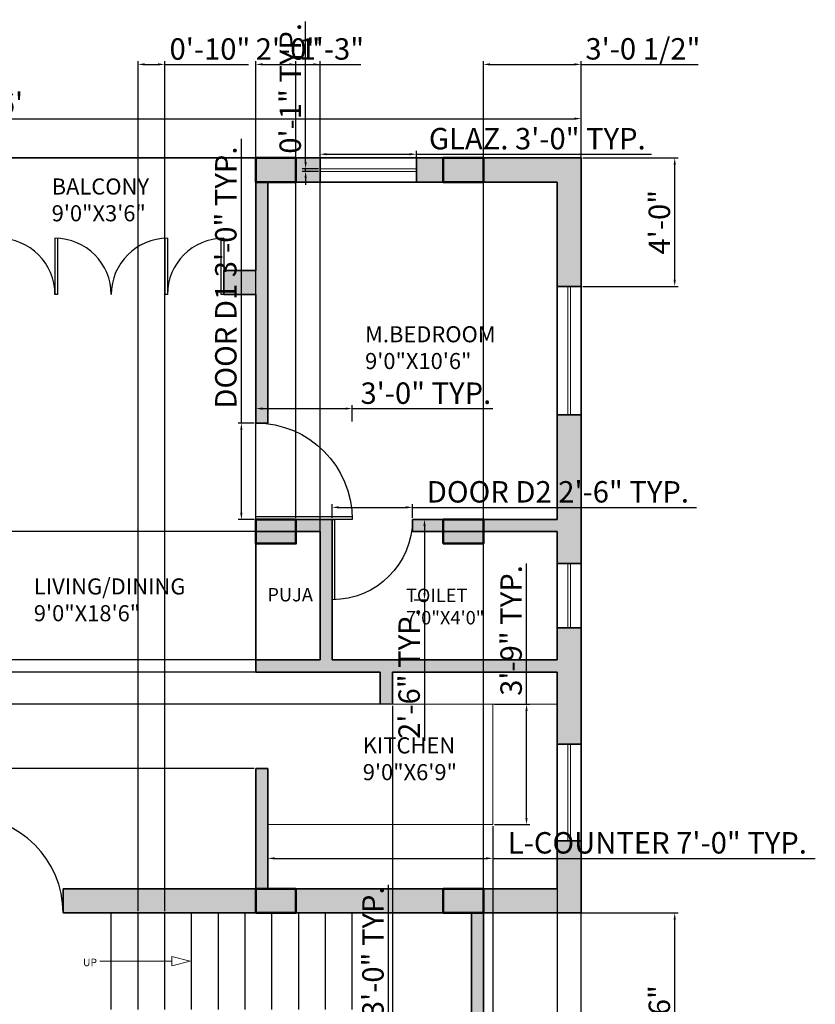
# Model space of a CAD drawing. Units: inches. Extents: x 3010 to 3575, y 2253 to 2995.
# Tile 4 of 4: x 3278 to 3575, y 2627 to 2995. Entities that reach past the tile are written whole.
import ezdxf

# ---------------------------------------------------------------- set-up
doc = ezdxf.new("R2010")
doc.units = ezdxf.units.IN
for name, color, linetype, lineweight in [('A-ANNO-DIMS', 2, 'Continuous', 18), ('A-ANNO-SYMB', 7, 'Continuous', 18), ('A-ANNO-TEXT', 7, 'Continuous', 18), ('A-AREA-IDEN', 7, 'Continuous', 18), ('A-COLS', 7, 'Continuous', 50), ('A-COLS-PATT', 1, 'Continuous', 13), ('A-DOOR', 3, 'Continuous', 25), ('A-FLOR-FIXT', 8, 'Continuous', 18), ('A-FLOR-STRS', 7, 'Continuous', 25), ('A-GLAZ', 4, 'Continuous', 18), ('A-WALL', 7, 'Continuous', 35)]:
    doc.layers.add(name, color=color, linetype=linetype, lineweight=lineweight)
doc.layers.add('A-WALL-PATT', color=9, linetype='Continuous', lineweight=13, true_color=0xc7c8ca)
doc.styles.get("Standard").update_dxf_attribs({"font": 'arial.ttf'})
doc.dimstyles.new('ISO-25', dxfattribs={"dimtxt": 8, "dimasz": 2.5, "dimexe": 1.25, "dimexo": 0.625, "dimtad": 1, "dimdec": 1, "dimlunit": 3, "dimtxsty": 'Standard', "dimcen": 2.5, "dimadec": 0, "dimazin": 0, "dimtfac": 1, "dimtdec": 1, "dimtmove": 0, "dimatfit": 3, "dimfxl": 1, "dimarcsym": 0})

# ---------------------------------------------------------------- blocks, each defined once
blk = doc.blocks.new('*D1')
at = {"layer": 'A-ANNO-DIMS', "color": 0, "lineweight": -2, "transparency": 16777216}
for p, q in [((3055.45, 2944.01), (3055.45, 2959.31)), ((3057.95, 2958.06), (3484.95, 2958.06)), ((3487.45, 2944.01), (3487.45, 2959.31))]:
    blk.add_line(p, q, dxfattribs=at)
at = {"layer": 'A-ANNO-DIMS', "color": 0, "transparency": 16777216}
for points in [[(3057.95, 2958.48), (3057.95, 2957.65), (3055.45, 2958.06)], [(3484.95, 2958.48), (3484.95, 2957.65), (3487.45, 2958.06)]]:
    blk.add_solid(points, dxfattribs=at)
at = {"layer": 'Defpoints', "color": 0, "transparency": 16777216}
for p in [(3487.45, 2958.06), (3055.45, 2943.38), (3487.45, 2943.38)]:
    blk.add_point(p, dxfattribs=at)
at = {"layer": 'A-ANNO-DIMS', "color": 0, "transparency": 16777216, "insert": (3271.45, 2962.78), "char_height": 8, "attachment_point": 5}
blk.add_mtext("36'", dxfattribs=at)
blk = doc.blocks.new("D2 2'6")
for p, q in [((0, 30), (0, 0)), ((1, 30), (1, 0)), ((0, 0), (1, 0))]:
    blk.add_line(p, q)
blk.add_arc((0, 0), 30, 0, 90)
blk = doc.blocks.new("D1 3'")
for p, q in [((0, 36), (0, 0)), ((1, 36), (1, 0)), ((0, 0), (1, 0))]:
    blk.add_line(p, q)
blk.add_arc((0, 0), 36, 0, 90)
blk = doc.blocks.new('FLOD D')
for p, q in [((3539.49, 2401.61), (3539.49, 2380.61)), ((3540.49, 2401.61), (3540.49, 2380.61)), ((3560.49, 2401.61), (3560.49, 2380.61)), ((3561.49, 2401.61), (3561.49, 2380.61)), ((3601.49, 2401.61), (3601.49, 2380.61)), ((3602.49, 2401.61), (3602.49, 2380.61)), ((3622.49, 2401.61), (3622.49, 2380.61)), ((3623.49, 2401.61), (3623.49, 2380.61)), ((3540.49, 2380.61), (3539.49, 2380.61)), ((3561.49, 2380.61), (3560.49, 2380.61)), ((3602.49, 2380.61), (3601.49, 2380.61)), ((3623.49, 2380.61), (3622.49, 2380.61))]:
    blk.add_line(p, q)
for centre, start, end in [((3539.49, 2380.61), 0, 90), ((3560.49, 2380.61), 0, 90), ((3602.49, 2380.61), 90, 180), ((3623.49, 2380.61), 90, 180)]:
    blk.add_arc(centre, 21, start, end)
blk = doc.blocks.new('GLAZING-24IN')
for p, q in [((24, 1), (0, 1)), ((24, 0), (0, 0))]:
    blk.add_line(p, q)
blk = doc.blocks.new('GLAZING-36IN')
for p, q in [((36, 1), (0, 1)), ((36, 0), (0, 0))]:
    blk.add_line(p, q)
blk = doc.blocks.new('GLAZING-48IN')
for p, q in [((48, 1), (0, 1)), ((48, 0), (0, 0))]:
    blk.add_line(p, q)
blk = doc.blocks.new('STAIR-FLIGHT-36IN')
for p, q in [((0, 0), (0, 36)), ((10, 0), (10, 36)), ((20, 0), (20, 36)), ((30, 0), (30, 36)), ((40, 0), (40, 36)), ((50, 0), (50, 36)), ((60, 0), (60, 36)), ((70, 0), (70, 36)), ((80, 0), (80, 36)), ((90, 0), (90, 36))]:
    blk.add_line(p, q)
blk = doc.blocks.new('STAIR-DIRECTION-ARROW')
blk.add_line((0, 1.77), (26.94, 1.77))
blk.add_lwpolyline([(33.73, 1.77), (26.94, 3.54), (26.94, 0)], close=True)
blk = doc.blocks.new('KITCHEN-COUNTER-L')
for p, q in [((84, 45), (84, 0)), ((84, 0), (0, 0))]:
    blk.add_line(p, q)
blk = doc.blocks.new('*D15')
at = {"layer": 'A-ANNO-DIMS', "color": 0, "lineweight": -2, "transparency": 16777216}
for p, q in [((3389.94, 2940.01), (3389.94, 2946.03)), ((3425.94, 2940.01), (3425.94, 2946.03)), ((3392.44, 2944.78), (3423.44, 2944.78)), ((3425.94, 2944.78), (3513.72, 2944.78))]:
    blk.add_line(p, q, dxfattribs=at)
at = {"layer": 'A-ANNO-DIMS', "color": 0, "transparency": 16777216}
for points in [[(3392.44, 2945.2), (3392.44, 2944.37), (3389.94, 2944.78)], [(3423.44, 2945.2), (3423.44, 2944.37), (3425.94, 2944.78)]]:
    blk.add_solid(points, dxfattribs=at)
at = {"layer": 'Defpoints', "color": 0, "transparency": 16777216}
for p in [(3425.94, 2944.78), (3389.94, 2939.38), (3425.94, 2939.38)]:
    blk.add_point(p, dxfattribs=at)
at = {"layer": 'A-ANNO-DIMS', "color": 0, "transparency": 16777216, "insert": (3471.08, 2949.55), "char_height": 8, "attachment_point": 5}
blk.add_mtext('GLAZ. 3\'-0" TYP.', dxfattribs=at)
blk = doc.blocks.new('*D16')
at = {"layer": 'A-ANNO-DIMS', "color": 0, "lineweight": -2, "transparency": 16777216}
for p, q in [((3384.54, 2941.88), (3384.54, 2994.4)), ((3389.31, 2939.38), (3383.29, 2939.38)), ((3389.31, 2938.38), (3383.29, 2938.38)), ((3384.54, 2938.38), (3384.54, 2939.38)), ((3384.54, 2935.88), (3384.54, 2933.38))]:
    blk.add_line(p, q, dxfattribs=at)
at = {"layer": 'A-ANNO-DIMS', "color": 0, "transparency": 16777216}
for points in [[(3384.12, 2941.88), (3384.95, 2941.88), (3384.54, 2939.38)], [(3384.12, 2935.88), (3384.95, 2935.88), (3384.54, 2938.38)]]:
    blk.add_solid(points, dxfattribs=at)
at = {"layer": 'Defpoints', "color": 0, "transparency": 16777216}
for p in [(3384.54, 2939.38), (3389.94, 2939.38), (3389.94, 2938.38)]:
    blk.add_point(p, dxfattribs=at)
at = {"layer": 'A-ANNO-DIMS', "color": 0, "transparency": 16777216, "insert": (3379.83, 2969.39), "char_height": 8, "attachment_point": 5, "rotation": 90}
blk.add_mtext('0\'-1" TYP.', dxfattribs=at)
blk = doc.blocks.new('*D23')
at = {"layer": 'A-ANNO-DIMS', "color": 0, "lineweight": -2, "transparency": 16777216}
for p, q in [((3360.55, 2844.38), (3360.55, 2950.52)), ((3365.32, 2844.38), (3359.3, 2844.38)), ((3360.55, 2810.88), (3360.55, 2841.88)), ((3365.32, 2808.38), (3359.3, 2808.38))]:
    blk.add_line(p, q, dxfattribs=at)
at = {"layer": 'A-ANNO-DIMS', "color": 0, "transparency": 16777216}
for points in [[(3360.13, 2841.88), (3360.96, 2841.88), (3360.55, 2844.38)], [(3360.13, 2810.88), (3360.96, 2810.88), (3360.55, 2808.38)]]:
    blk.add_solid(points, dxfattribs=at)
at = {"layer": 'Defpoints', "color": 0, "transparency": 16777216}
for p in [(3360.55, 2844.38), (3365.95, 2844.38), (3365.95, 2808.38)]:
    blk.add_point(p, dxfattribs=at)
at = {"layer": 'A-ANNO-DIMS', "color": 0, "transparency": 16777216, "insert": (3355.78, 2898.7), "char_height": 8, "attachment_point": 5, "rotation": 90}
blk.add_mtext('DOOR D1 3\'-0" TYP.', dxfattribs=at)
blk = doc.blocks.new('*D24')
at = {"layer": 'A-ANNO-DIMS', "color": 0, "lineweight": -2, "transparency": 16777216}
for p, q in [((3365.95, 2845.01), (3365.95, 2851.03)), ((3401.95, 2845.01), (3401.95, 2851.03)), ((3368.45, 2849.78), (3399.45, 2849.78)), ((3401.95, 2849.78), (3454.45, 2849.78))]:
    blk.add_line(p, q, dxfattribs=at)
at = {"layer": 'A-ANNO-DIMS', "color": 0, "transparency": 16777216}
for points in [[(3368.45, 2850.2), (3368.45, 2849.37), (3365.95, 2849.78)], [(3399.45, 2850.2), (3399.45, 2849.37), (3401.95, 2849.78)]]:
    blk.add_solid(points, dxfattribs=at)
at = {"layer": 'Defpoints', "color": 0, "transparency": 16777216}
for p in [(3401.95, 2849.78), (3365.95, 2844.38), (3401.95, 2844.38)]:
    blk.add_point(p, dxfattribs=at)
at = {"layer": 'A-ANNO-DIMS', "color": 0, "transparency": 16777216, "insert": (3429.45, 2854.5), "char_height": 8, "attachment_point": 5}
blk.add_mtext('3\'-0" TYP.', dxfattribs=at)
blk = doc.blocks.new('*D25')
at = {"layer": 'A-ANNO-DIMS', "color": 0, "lineweight": -2, "transparency": 16777216}
for p, q in [((3394.45, 2809.01), (3394.45, 2814.13)), ((3424.45, 2809.01), (3424.45, 2814.13)), ((3396.95, 2812.88), (3421.95, 2812.88)), ((3424.45, 2812.88), (3530.59, 2812.88))]:
    blk.add_line(p, q, dxfattribs=at)
at = {"layer": 'A-ANNO-DIMS', "color": 0, "transparency": 16777216}
for points in [[(3396.95, 2813.3), (3396.95, 2812.47), (3394.45, 2812.88)], [(3421.95, 2813.3), (3421.95, 2812.47), (3424.45, 2812.88)]]:
    blk.add_solid(points, dxfattribs=at)
at = {"layer": 'Defpoints', "color": 0, "transparency": 16777216}
for p in [(3424.45, 2812.88), (3394.45, 2808.38), (3424.45, 2808.38)]:
    blk.add_point(p, dxfattribs=at)
at = {"layer": 'A-ANNO-DIMS', "color": 0, "transparency": 16777216, "insert": (3478.77, 2817.65), "char_height": 8, "attachment_point": 5}
blk.add_mtext('DOOR D2 2\'-6" TYP.', dxfattribs=at)
blk = doc.blocks.new('*D26')
at = {"layer": 'A-ANNO-DIMS', "color": 0, "lineweight": -2, "transparency": 16777216}
for p, q in [((3425.07, 2808.38), (3430.2, 2808.38)), ((3428.95, 2805.88), (3428.95, 2780.88)), ((3425.07, 2778.38), (3430.2, 2778.38)), ((3428.95, 2778.38), (3428.95, 2725.73))]:
    blk.add_line(p, q, dxfattribs=at)
at = {"layer": 'A-ANNO-DIMS', "color": 0, "transparency": 16777216}
for points in [[(3428.53, 2805.88), (3429.36, 2805.88), (3428.95, 2808.38)], [(3428.53, 2780.88), (3429.36, 2780.88), (3428.95, 2778.38)]]:
    blk.add_solid(points, dxfattribs=at)
at = {"layer": 'Defpoints', "color": 0, "transparency": 16777216}
for p in [(3424.45, 2808.38), (3424.45, 2778.38), (3428.95, 2778.38)]:
    blk.add_point(p, dxfattribs=at)
at = {"layer": 'A-ANNO-DIMS', "color": 0, "transparency": 16777216, "insert": (3424.24, 2750.81), "char_height": 8, "attachment_point": 5, "rotation": 90}
blk.add_mtext('2\'-6" TYP.', dxfattribs=at)
blk = doc.blocks.new('*D31')
at = {"layer": 'A-ANNO-DIMS', "color": 0, "lineweight": -2, "transparency": 16777216}
for p, q in [((3370.45, 2693.76), (3370.45, 2680.53)), ((3454.45, 2693.76), (3454.45, 2680.53)), ((3372.95, 2681.78), (3451.95, 2681.78)), ((3454.45, 2681.78), (3574.9, 2681.78))]:
    blk.add_line(p, q, dxfattribs=at)
at = {"layer": 'A-ANNO-DIMS', "color": 0, "transparency": 16777216}
for points in [[(3372.95, 2682.2), (3372.95, 2681.37), (3370.45, 2681.78)], [(3451.95, 2682.2), (3451.95, 2681.37), (3454.45, 2681.78)]]:
    blk.add_solid(points, dxfattribs=at)
at = {"layer": 'Defpoints', "color": 0, "transparency": 16777216}
for p in [(3370.45, 2694.38), (3454.45, 2694.38), (3454.45, 2681.78)]:
    blk.add_point(p, dxfattribs=at)
at = {"layer": 'A-ANNO-DIMS', "color": 0, "transparency": 16777216, "insert": (3515.92, 2686.55), "char_height": 8, "attachment_point": 5}
blk.add_mtext('L-COUNTER 7\'-0" TYP.', dxfattribs=at)
blk = doc.blocks.new('*D32')
at = {"layer": 'A-ANNO-DIMS', "color": 0, "lineweight": -2, "transparency": 16777216}
for p, q in [((3467.05, 2739.38), (3467.05, 2791.89)), ((3455.07, 2739.38), (3468.3, 2739.38)), ((3467.05, 2696.88), (3467.05, 2736.88)), ((3455.07, 2694.38), (3468.3, 2694.38))]:
    blk.add_line(p, q, dxfattribs=at)
at = {"layer": 'A-ANNO-DIMS', "color": 0, "transparency": 16777216}
for points in [[(3466.63, 2736.88), (3467.46, 2736.88), (3467.05, 2739.38)], [(3466.63, 2696.88), (3467.46, 2696.88), (3467.05, 2694.38)]]:
    blk.add_solid(points, dxfattribs=at)
at = {"layer": 'Defpoints', "color": 0, "transparency": 16777216}
for p in [(3454.45, 2739.38), (3467.05, 2739.38), (3454.45, 2694.38)]:
    blk.add_point(p, dxfattribs=at)
at = {"layer": 'A-ANNO-DIMS', "color": 0, "transparency": 16777216, "insert": (3462.33, 2766.89), "char_height": 8, "attachment_point": 5, "rotation": 90}
blk.add_mtext('3\'-9" TYP.', dxfattribs=at)
blk = doc.blocks.new('*D34')
at = {"layer": 'A-ANNO-DIMS', "color": 0, "lineweight": -2, "transparency": 16777216}
for p, q in [((3415.45, 2619.38), (3415.45, 2671.89)), ((3402.57, 2619.38), (3416.7, 2619.38)), ((3415.45, 2585.88), (3415.45, 2616.88)), ((3402.57, 2583.38), (3416.7, 2583.38))]:
    blk.add_line(p, q, dxfattribs=at)
at = {"layer": 'A-ANNO-DIMS', "color": 0, "transparency": 16777216}
for points in [[(3415.03, 2616.88), (3415.86, 2616.88), (3415.45, 2619.38)], [(3415.03, 2585.88), (3415.86, 2585.88), (3415.45, 2583.38)]]:
    blk.add_solid(points, dxfattribs=at)
at = {"layer": 'Defpoints', "color": 0, "transparency": 16777216}
for p in [(3401.95, 2619.38), (3415.45, 2619.38), (3401.95, 2583.38)]:
    blk.add_point(p, dxfattribs=at)
at = {"layer": 'A-ANNO-DIMS', "color": 0, "transparency": 16777216, "insert": (3410.73, 2646.89), "char_height": 8, "attachment_point": 5, "rotation": 90}
blk.add_mtext('3\'-0" TYP.', dxfattribs=at)
blk = doc.blocks.new('*D37')
at = {"layer": 'A-ANNO-DIMS', "color": 0, "lineweight": -2, "transparency": 16777216}
for p, q in [((3447.07, 2661.38), (3523.65, 2661.38)), ((3522.4, 2585.88), (3522.4, 2658.88)), ((3447.07, 2583.38), (3523.65, 2583.38))]:
    blk.add_line(p, q, dxfattribs=at)
at = {"layer": 'A-ANNO-DIMS', "color": 0, "transparency": 16777216}
for points in [[(3521.98, 2658.88), (3522.81, 2658.88), (3522.4, 2661.38)], [(3521.98, 2585.88), (3522.81, 2585.88), (3522.4, 2583.38)]]:
    blk.add_solid(points, dxfattribs=at)
at = {"layer": 'Defpoints', "color": 0, "transparency": 16777216}
for p in [(3446.45, 2661.38), (3522.4, 2661.38), (3446.45, 2583.38)]:
    blk.add_point(p, dxfattribs=at)
at = {"layer": 'A-ANNO-DIMS', "color": 0, "transparency": 16777216, "insert": (3517.69, 2622.38), "char_height": 8, "attachment_point": 5, "rotation": 90}
blk.add_mtext('6\'-6"', dxfattribs=at)
blk = doc.blocks.new('*D38')
at = {"layer": 'A-ANNO-DIMS', "color": 0, "lineweight": -2, "transparency": 16777216}
for p, q in [((3321.95, 2662.01), (3321.95, 2979.58)), ((3331.95, 2662.01), (3331.95, 2979.58)), ((3324.45, 2978.33), (3329.45, 2978.33)), ((3331.95, 2978.33), (3363.18, 2978.33))]:
    blk.add_line(p, q, dxfattribs=at)
at = {"layer": 'A-ANNO-DIMS', "color": 0, "transparency": 16777216}
for points in [[(3324.45, 2978.75), (3324.45, 2977.92), (3321.95, 2978.33)], [(3329.45, 2978.75), (3329.45, 2977.92), (3331.95, 2978.33)]]:
    blk.add_solid(points, dxfattribs=at)
at = {"layer": 'Defpoints', "color": 0, "transparency": 16777216}
for p in [(3331.95, 2978.33), (3321.95, 2661.38), (3331.95, 2661.38)]:
    blk.add_point(p, dxfattribs=at)
at = {"layer": 'A-ANNO-DIMS', "color": 0, "transparency": 16777216, "insert": (3348.81, 2983.04), "char_height": 8, "attachment_point": 5}
blk.add_mtext('0\'-10"', dxfattribs=at)
blk = doc.blocks.new('*D39')
at = {"layer": 'A-ANNO-DIMS', "color": 0, "lineweight": -2, "transparency": 16777216}
for p, q in [((3365.95, 2756.51), (3365.95, 2979.58)), ((3389.95, 2756.51), (3389.95, 2979.58)), ((3368.45, 2978.33), (3387.45, 2978.33))]:
    blk.add_line(p, q, dxfattribs=at)
at = {"layer": 'A-ANNO-DIMS', "color": 0, "transparency": 16777216}
for points in [[(3368.45, 2978.75), (3368.45, 2977.92), (3365.95, 2978.33)], [(3387.45, 2978.75), (3387.45, 2977.92), (3389.95, 2978.33)]]:
    blk.add_solid(points, dxfattribs=at)
at = {"layer": 'Defpoints', "color": 0, "transparency": 16777216}
for p in [(3389.95, 2978.33), (3365.95, 2755.88), (3389.95, 2755.88)]:
    blk.add_point(p, dxfattribs=at)
at = {"layer": 'A-ANNO-DIMS', "color": 0, "transparency": 16777216, "insert": (3377.95, 2983.04), "char_height": 8, "attachment_point": 5}
blk.add_mtext('2\'-0"', dxfattribs=at)
blk = doc.blocks.new('*D40')
at = {"layer": 'A-ANNO-DIMS', "color": 0, "lineweight": -2, "transparency": 16777216}
for p, q in [((3389.32, 2803.88), (3019.25, 2803.88)), ((3020.5, 2758.38), (3020.5, 2801.38)), ((3389.32, 2755.88), (3019.25, 2755.88))]:
    blk.add_line(p, q, dxfattribs=at)
at = {"layer": 'A-ANNO-DIMS', "color": 0, "transparency": 16777216}
for points in [[(3020.08, 2801.38), (3020.91, 2801.38), (3020.5, 2803.88)], [(3020.08, 2758.38), (3020.91, 2758.38), (3020.5, 2755.88)]]:
    blk.add_solid(points, dxfattribs=at)
at = {"layer": 'Defpoints', "color": 0, "transparency": 16777216}
for p in [(3020.5, 2803.88), (3389.95, 2803.88), (3389.95, 2755.88)]:
    blk.add_point(p, dxfattribs=at)
at = {"layer": 'A-ANNO-DIMS', "color": 0, "transparency": 16777216, "insert": (3015.79, 2779.88), "char_height": 8, "attachment_point": 5, "rotation": 90}
blk.add_mtext('4\'-0"', dxfattribs=at)
blk = doc.blocks.new('*D41')
at = {"layer": 'A-ANNO-DIMS', "color": 0, "lineweight": -2, "transparency": 16777216}
for p, q in [((3454.45, 2693.76), (3454.45, 2259.18)), ((3478.45, 2669.76), (3478.45, 2259.18)), ((3456.95, 2260.43), (3475.95, 2260.43))]:
    blk.add_line(p, q, dxfattribs=at)
at = {"layer": 'A-ANNO-DIMS', "color": 0, "transparency": 16777216}
for points in [[(3456.95, 2260.85), (3456.95, 2260.02), (3454.45, 2260.43)], [(3475.95, 2260.85), (3475.95, 2260.02), (3478.45, 2260.43)]]:
    blk.add_solid(points, dxfattribs=at)
at = {"layer": 'Defpoints', "color": 0, "transparency": 16777216}
for p in [(3454.45, 2694.38), (3478.45, 2670.38), (3478.45, 2260.43)]:
    blk.add_point(p, dxfattribs=at)
at = {"layer": 'A-ANNO-DIMS', "color": 0, "transparency": 16777216, "insert": (3466.45, 2265.14), "char_height": 8, "attachment_point": 5}
blk.add_mtext('2\'-0"', dxfattribs=at)
blk = doc.blocks.new('*D42')
at = {"layer": 'A-ANNO-DIMS', "color": 0, "lineweight": -2, "transparency": 16777216}
for p, q in [((3365.32, 2751.38), (3019.25, 2751.38)), ((3020.5, 2717.88), (3020.5, 2748.88)), ((3365.32, 2715.38), (3019.25, 2715.38))]:
    blk.add_line(p, q, dxfattribs=at)
at = {"layer": 'A-ANNO-DIMS', "color": 0, "transparency": 16777216}
for points in [[(3020.08, 2748.88), (3020.91, 2748.88), (3020.5, 2751.38)], [(3020.08, 2717.88), (3020.91, 2717.88), (3020.5, 2715.38)]]:
    blk.add_solid(points, dxfattribs=at)
at = {"layer": 'Defpoints', "color": 0, "transparency": 16777216}
for p in [(3020.5, 2751.38), (3365.95, 2751.38), (3365.95, 2715.38)]:
    blk.add_point(p, dxfattribs=at)
at = {"layer": 'A-ANNO-DIMS', "color": 0, "transparency": 16777216, "insert": (3015.78, 2733.38), "char_height": 8, "attachment_point": 5, "rotation": 90}
blk.add_mtext('3\'-0"', dxfattribs=at)
blk = doc.blocks.new('*D43')
at = {"layer": 'A-ANNO-DIMS', "color": 0, "lineweight": -2, "transparency": 16777216}
for p, q in [((3020.5, 2751.38), (3020.5, 2775.65)), ((3411.82, 2751.38), (3019.25, 2751.38)), ((3020.5, 2741.88), (3020.5, 2748.88)), ((3416.32, 2739.38), (3019.25, 2739.38))]:
    blk.add_line(p, q, dxfattribs=at)
at = {"layer": 'A-ANNO-DIMS', "color": 0, "transparency": 16777216}
for points in [[(3020.08, 2748.88), (3020.91, 2748.88), (3020.5, 2751.38)], [(3020.08, 2741.88), (3020.91, 2741.88), (3020.5, 2739.38)]]:
    blk.add_solid(points, dxfattribs=at)
at = {"layer": 'Defpoints', "color": 0, "transparency": 16777216}
for p in [(3020.5, 2751.38), (3412.45, 2751.38), (3416.95, 2739.38)]:
    blk.add_point(p, dxfattribs=at)
at = {"layer": 'A-ANNO-DIMS', "color": 0, "transparency": 16777216, "insert": (3015.79, 2764.76), "char_height": 8, "attachment_point": 5, "rotation": 90}
blk.add_mtext('1\'-0"', dxfattribs=at)
blk = doc.blocks.new('*D44')
at = {"layer": 'A-ANNO-DIMS', "color": 0, "lineweight": -2, "transparency": 16777216}
for p, q in [((3416.95, 2738.76), (3416.95, 2259.18)), ((3478.45, 2738.76), (3478.45, 2259.18)), ((3419.45, 2260.43), (3475.95, 2260.43))]:
    blk.add_line(p, q, dxfattribs=at)
at = {"layer": 'A-ANNO-DIMS', "color": 0, "transparency": 16777216}
for points in [[(3419.45, 2260.85), (3419.45, 2260.02), (3416.95, 2260.43)], [(3475.95, 2260.85), (3475.95, 2260.02), (3478.45, 2260.43)]]:
    blk.add_solid(points, dxfattribs=at)
at = {"layer": 'Defpoints', "color": 0, "transparency": 16777216}
for p in [(3416.95, 2739.38), (3478.45, 2739.38), (3478.45, 2260.43)]:
    blk.add_point(p, dxfattribs=at)
at = {"layer": 'A-ANNO-DIMS', "color": 0, "transparency": 16777216, "insert": (3447.7, 2265.19), "char_height": 8, "attachment_point": 5}
blk.add_mtext('5\'-1 1/2"', dxfattribs=at)
blk = doc.blocks.new('*D45')
at = {"layer": 'A-ANNO-DIMS', "color": 0, "lineweight": -2, "transparency": 16777216}
for p, q in [((3365.95, 2809.01), (3365.95, 2979.58)), ((3380.95, 2809.01), (3380.95, 2979.58)), ((3368.45, 2978.33), (3378.45, 2978.33)), ((3380.95, 2978.33), (3405.21, 2978.33))]:
    blk.add_line(p, q, dxfattribs=at)
at = {"layer": 'A-ANNO-DIMS', "color": 0, "transparency": 16777216}
for points in [[(3368.45, 2978.75), (3368.45, 2977.92), (3365.95, 2978.33)], [(3378.45, 2978.75), (3378.45, 2977.92), (3380.95, 2978.33)]]:
    blk.add_solid(points, dxfattribs=at)
at = {"layer": 'Defpoints', "color": 0, "transparency": 16777216}
for p in [(3380.95, 2978.33), (3365.95, 2808.38), (3380.95, 2808.38)]:
    blk.add_point(p, dxfattribs=at)
at = {"layer": 'A-ANNO-DIMS', "color": 0, "transparency": 16777216, "insert": (3394.33, 2983.05), "char_height": 8, "attachment_point": 5}
blk.add_mtext('1\'-3"', dxfattribs=at)
blk = doc.blocks.new('*D50')
at = {"layer": 'A-ANNO-DIMS', "color": 0, "lineweight": -2, "transparency": 16777216}
for p, q in [((3450.95, 2584.01), (3450.95, 2979.58)), ((3487.45, 2584.01), (3487.45, 2979.58)), ((3453.45, 2978.33), (3484.95, 2978.33)), ((3487.45, 2978.33), (3531.1, 2978.33))]:
    blk.add_line(p, q, dxfattribs=at)
at = {"layer": 'A-ANNO-DIMS', "color": 0, "transparency": 16777216}
for points in [[(3453.45, 2978.75), (3453.45, 2977.92), (3450.95, 2978.33)], [(3484.95, 2978.75), (3484.95, 2977.92), (3487.45, 2978.33)]]:
    blk.add_solid(points, dxfattribs=at)
at = {"layer": 'Defpoints', "color": 0, "transparency": 16777216}
for p in [(3487.45, 2978.33), (3450.95, 2583.38), (3487.45, 2583.38)]:
    blk.add_point(p, dxfattribs=at)
at = {"layer": 'A-ANNO-DIMS', "color": 0, "transparency": 16777216, "insert": (3510.52, 2983.1), "char_height": 8, "attachment_point": 5}
blk.add_mtext('3\'-0 1/2"', dxfattribs=at)
blk = doc.blocks.new('*D54')
at = {"layer": 'A-ANNO-DIMS', "color": 0, "lineweight": -2, "transparency": 16777216}
for p, q in [((3488.07, 2943.38), (3523.65, 2943.38)), ((3522.4, 2897.88), (3522.4, 2940.88)), ((3488.07, 2895.38), (3523.65, 2895.38))]:
    blk.add_line(p, q, dxfattribs=at)
at = {"layer": 'A-ANNO-DIMS', "color": 0, "transparency": 16777216}
for points in [[(3521.98, 2940.88), (3522.81, 2940.88), (3522.4, 2943.38)], [(3521.98, 2897.88), (3522.81, 2897.88), (3522.4, 2895.38)]]:
    blk.add_solid(points, dxfattribs=at)
at = {"layer": 'Defpoints', "color": 0, "transparency": 16777216}
for p in [(3487.45, 2943.38), (3522.4, 2943.38), (3487.45, 2895.38)]:
    blk.add_point(p, dxfattribs=at)
at = {"layer": 'A-ANNO-DIMS', "color": 0, "transparency": 16777216, "insert": (3517.69, 2919.38), "char_height": 8, "attachment_point": 5, "rotation": 90}
blk.add_mtext('4\'-0"', dxfattribs=at)

msp = doc.modelspace()

# ---------------------------------------------------------------- hatches: boundary and pattern name
at = {"layer": 'A-COLS-PATT'}
h = msp.add_hatch(color=256, dxfattribs=at)
h.dxf.hatch_style = 1
h.paths.add_polyline_path([(3380.95, 2934.38), (3380.95, 2943.38), (3365.95, 2943.38), (3365.95, 2934.38)])
h = msp.add_hatch(color=256, dxfattribs=at)
h.dxf.hatch_style = 1
h.paths.add_polyline_path([(3450.95, 2934.38), (3450.95, 2943.38), (3435.95, 2943.38), (3435.95, 2934.38)])
h = msp.add_hatch(color=256, dxfattribs=at)
h.dxf.hatch_style = 1
h.paths.add_polyline_path([(3380.95, 2799.38), (3380.95, 2808.38), (3365.95, 2808.38), (3365.95, 2799.38)])
h = msp.add_hatch(color=256, dxfattribs=at)
h.dxf.hatch_style = 1
h.paths.add_polyline_path([(3450.95, 2799.38), (3450.95, 2808.38), (3435.95, 2808.38), (3435.95, 2799.38)])
h = msp.add_hatch(color=256, dxfattribs=at)
h.dxf.hatch_style = 1
h.paths.add_polyline_path([(3380.95, 2661.38), (3380.95, 2670.38), (3365.95, 2670.38), (3365.95, 2661.38)])
h = msp.add_hatch(color=256, dxfattribs=at)
h.dxf.hatch_style = 1
h.paths.add_polyline_path([(3450.95, 2661.38), (3450.95, 2670.38), (3435.95, 2670.38), (3435.95, 2661.38)])
at = {"layer": 'A-WALL-PATT', "transparency": 33554687}
h = msp.add_hatch(color=256, dxfattribs=at)
h.dxf.hatch_style = 1
h.paths.add_polyline_path([(3064.45, 2499.38), (3055.45, 2499.38), (3055.45, 2457.38), (3064.45, 2457.38)])
h.paths.add_polyline_path([(3091.95, 2421.38), (3055.45, 2421.38), (3055.45, 2382.38), (3064.45, 2382.38), (3064.45, 2412.38), (3091.95, 2412.38)])
h.paths.add_polyline_path([(3248.95, 2421.38), (3176.95, 2421.38), (3176.95, 2464.88), (3194.99, 2464.88), (3194.99, 2473.88), (3176.95, 2473.88), (3176.95, 2551.88), (3172.45, 2551.88), (3172.45, 2515.88), (3172.45, 2421.38), (3106.95, 2421.38), (3106.95, 2412.38), (3248.95, 2412.38)])
h.paths.add_polyline_path([(3064.45, 2346.38), (3055.45, 2346.38), (3055.45, 2295.38), (3091.95, 2295.38), (3091.95, 2304.38), (3064.45, 2304.38)])
h.paths.add_polyline_path([(3129.95, 2304.38), (3106.95, 2304.38), (3106.95, 2295.38), (3129.95, 2295.38)])
h.paths.add_polyline_path([(3211.45, 2304.38), (3193.45, 2304.38), (3193.45, 2376.88), (3188.95, 2376.88), (3188.95, 2304.38), (3165.95, 2304.38), (3165.95, 2295.38), (3211.45, 2295.38)])
h.paths.add_polyline_path([(3269.95, 2346.38), (3257.95, 2346.38), (3257.95, 2376.88), (3223.45, 2376.88), (3223.45, 2371.88), (3253.45, 2371.88), (3253.45, 2304.38), (3257.95, 2304.38), (3257.95, 2337.38), (3269.95, 2337.38)])
h.paths.add_polyline_path([(3242.95, 2304.38), (3235.45, 2304.38), (3235.45, 2295.38), (3242.95, 2295.38)])
h.paths.add_polyline_path([(3370.45, 2346.38), (3353.95, 2346.38), (3353.95, 2337.38), (3365.95, 2337.38), (3365.95, 2304.38), (3370.45, 2304.38)])
h.paths.add_polyline_path([(3389.94, 2304.38), (3380.95, 2304.38), (3380.95, 2295.38), (3389.94, 2295.38)], flags=17)
h.paths.add_polyline_path([(3435.95, 2304.38), (3425.94, 2304.38), (3425.94, 2295.38), (3435.95, 2295.38)], flags=17)
h.paths.add_polyline_path([(3487.45, 2401.88), (3478.45, 2401.88), (3478.45, 2389.88), (3394.45, 2389.88), (3394.45, 2442.38), (3380.95, 2442.38), (3380.95, 2437.88), (3389.95, 2437.88), (3389.95, 2389.88), (3365.95, 2389.88), (3365.95, 2385.38), (3412.45, 2385.38), (3412.45, 2373.38), (3416.95, 2373.38), (3416.95, 2385.38), (3478.45, 2385.38), (3478.45, 2304.38), (3450.95, 2304.38), (3450.95, 2295.38), (3487.45, 2295.38)])
h.paths.add_polyline_path([(3487.45, 2478.38), (3478.45, 2478.38), (3478.45, 2442.38), (3450.95, 2442.38), (3450.95, 2437.88), (3478.45, 2437.88), (3478.45, 2425.88), (3487.45, 2425.88)])
h.paths.add_polyline_path([(3435.95, 2442.38), (3424.45, 2442.38), (3424.45, 2437.88), (3435.95, 2437.88)], flags=17)
h.paths.add_polyline_path([(3248.95, 2592.38), (3221.95, 2592.38), (3172.45, 2592.38), (3172.45, 2587.88), (3248.95, 2587.88)])
h.paths.add_polyline_path([(3257.95, 2577.38), (3248.95, 2577.38), (3248.95, 2473.88), (3230.99, 2473.88), (3230.99, 2464.88), (3248.95, 2464.88), (3248.95, 2427.38), (3257.95, 2427.38)])
h.paths.add_polyline_path([(3365.95, 2583.38), (3293.95, 2583.38), (3293.95, 2574.38), (3365.95, 2574.38)])
h.paths.add_polyline_path([(3370.45, 2574.38), (3365.95, 2574.38), (3365.95, 2478.38), (3370.45, 2478.38)])
h.paths.add_polyline_path([(3435.95, 2583.38), (3380.95, 2583.38), (3380.95, 2574.38), (3435.95, 2574.38)])
h.paths.add_polyline_path([(3487.45, 2583.38), (3450.95, 2583.38), (3450.95, 2574.38), (3478.45, 2574.38), (3478.45, 2538.38), (3487.45, 2538.38)])
h.paths.add_polyline_path([(3064.45, 2551.88), (3055.45, 2551.88), (3055.45, 2535.38), (3136.45, 2535.38), (3136.45, 2557.88), (3131.95, 2557.88), (3131.95, 2539.88), (3064.45, 2539.88)])
h.paths.add_polyline_path([(3091.95, 2704.88), (3064.45, 2704.88), (3064.45, 2726.63), (3055.45, 2726.63), (3055.45, 2676.38), (3064.45, 2676.38), (3064.45, 2700.38), (3091.95, 2700.38)])
h.paths.add_polyline_path([(3064.45, 2616.38), (3055.45, 2616.38), (3055.45, 2575.88), (3064.45, 2575.88), (3064.45, 2587.88), (3091.95, 2587.88), (3091.95, 2592.38), (3064.45, 2592.38)])
h.paths.add_polyline_path([(3487.45, 2688.38), (3478.45, 2688.38), (3478.45, 2670.38), (3450.95, 2670.38), (3450.95, 2661.38), (3487.45, 2661.38)])
h.paths.add_polyline_path([(3450.95, 2661.38), (3446.45, 2661.38), (3446.45, 2583.38), (3450.95, 2583.38)])
h.paths.add_polyline_path([(3435.95, 2670.38), (3380.95, 2670.38), (3380.95, 2661.38), (3435.95, 2661.38)])
h.paths.add_polyline_path([(3365.95, 2670.38), (3293.95, 2670.38), (3293.95, 2661.38), (3365.95, 2661.38)])
h.paths.add_polyline_path([(3370.45, 2715.38), (3365.95, 2715.38), (3365.95, 2670.38), (3370.45, 2670.38)])
h.paths.add_polyline_path([(3257.95, 2700.38), (3248.95, 2700.38), (3248.95, 2628.38), (3257.95, 2628.38)])
h.paths.add_polyline_path([(3128.95, 2742.38), (3124.45, 2742.38), (3124.45, 2704.88), (3106.95, 2704.88), (3106.95, 2700.38), (3128.95, 2700.38)])
h.paths.add_polyline_path([(3248.95, 2704.88), (3164.95, 2704.88), (3164.95, 2700.38), (3248.95, 2700.38)])
h.paths.add_polyline_path([(3257.95, 2817.38), (3248.95, 2817.38), (3248.95, 2715.38), (3257.95, 2715.38)])
h.paths.add_polyline_path([(3128.95, 2781.38), (3055.45, 2781.38), (3055.45, 2750.63), (3064.45, 2750.63), (3064.45, 2772.38), (3128.95, 2772.38)])
h.paths.add_polyline_path([(3242.95, 2826.38), (3106.95, 2826.38), (3106.95, 2817.38), (3242.95, 2817.38)])
h.paths.add_polyline_path([(3091.95, 2826.38), (3064.45, 2826.38), (3064.45, 2856.38), (3055.45, 2856.38), (3055.45, 2817.38), (3091.95, 2817.38)])
h.paths.add_polyline_path([(3064.45, 2934.38), (3091.95, 2934.38), (3091.95, 2943.38), (3055.45, 2943.38), (3055.45, 2904.38), (3064.45, 2904.38)])
h.paths.add_polyline_path([(3140.95, 2943.38), (3106.95, 2943.38), (3106.95, 2934.38), (3140.95, 2934.38)])
h.paths.add_polyline_path([(3211.45, 2943.38), (3188.95, 2943.38), (3188.95, 2862.38), (3223.45, 2862.38), (3223.45, 2866.88), (3193.45, 2866.88), (3193.45, 2934.38), (3211.45, 2934.38)])
h.paths.add_polyline_path([(3257.95, 2934.38), (3253.45, 2934.38), (3253.45, 2862.38), (3257.95, 2862.38), (3257.95, 2892.38), (3269.95, 2892.38), (3269.95, 2901.38), (3257.95, 2901.38)])
h.paths.add_polyline_path([(3242.95, 2943.38), (3235.45, 2943.38), (3235.45, 2934.38), (3242.95, 2934.38)])
h.paths.add_polyline_path([(3370.45, 2934.38), (3365.95, 2934.38), (3365.95, 2901.38), (3353.95, 2901.38), (3353.95, 2892.38), (3365.95, 2892.38), (3365.95, 2844.38), (3370.45, 2844.38)])
h.paths.add_polyline_path([(3389.94, 2943.38), (3380.95, 2943.38), (3380.95, 2934.38), (3389.94, 2934.38)])
h.paths.add_polyline_path([(3435.95, 2943.38), (3425.94, 2943.38), (3425.94, 2934.38), (3435.95, 2934.38)])
h.paths.add_polyline_path([(3487.45, 2943.38), (3450.95, 2943.38), (3450.95, 2934.38), (3478.45, 2934.38), (3478.45, 2895.38), (3487.45, 2895.38)])
h.paths.add_polyline_path([(3487.45, 2847.38), (3478.45, 2847.38), (3478.45, 2808.38), (3450.95, 2808.38), (3450.95, 2803.88), (3478.45, 2803.88), (3478.45, 2791.88), (3487.45, 2791.88)])
h.paths.add_polyline_path([(3435.95, 2808.38), (3424.45, 2808.38), (3424.45, 2803.88), (3435.95, 2803.88)])
h.paths.add_polyline_path([(3487.45, 2767.88), (3478.45, 2767.88), (3478.45, 2755.88), (3394.45, 2755.88), (3394.45, 2808.38), (3380.95, 2808.38), (3380.95, 2803.88), (3389.95, 2803.88), (3389.95, 2755.88), (3365.95, 2755.88), (3365.95, 2751.38), (3412.45, 2751.38), (3412.45, 2739.38), (3416.95, 2739.38), (3416.95, 2751.38), (3478.45, 2751.38), (3478.45, 2724.38), (3487.45, 2724.38)])
h.paths.add_polyline_path([(3398.97, 2495.84), (3456.57, 2495.84), (3456.57, 2518.66), (3398.97, 2518.66)], flags=9)

# ---------------------------------------------------------------- linework, layer by layer
at = {"layer": 'A-COLS'}
for points in [[(3365.95, 2934.38), (3365.95, 2943.38), (3380.95, 2943.38), (3380.95, 2934.38)], [(3435.95, 2934.38), (3435.95, 2943.38), (3450.95, 2943.38), (3450.95, 2934.38)], [(3365.95, 2799.38), (3365.95, 2808.38), (3380.95, 2808.38), (3380.95, 2799.38)], [(3435.95, 2799.38), (3435.95, 2808.38), (3450.95, 2808.38), (3450.95, 2799.38)], [(3365.95, 2661.38), (3365.95, 2670.38), (3380.95, 2670.38), (3380.95, 2661.38)], [(3435.95, 2661.38), (3435.95, 2670.38), (3450.95, 2670.38), (3450.95, 2661.38)]]:
    msp.add_lwpolyline(points, close=True, dxfattribs=at)
at = {"layer": 'A-FLOR-FIXT'}
msp.add_line((3478.45, 2739.38), (3412.45, 2739.38), dxfattribs=at)
at = {"layer": 'A-WALL'}
for p, q in [((3055.45, 2943.38), (3487.45, 2943.38)), ((3365.95, 2943.38), (3365.95, 2901.38)), ((3389.94, 2943.38), (3389.94, 2934.38)), ((3425.94, 2943.38), (3425.94, 2934.38)), ((3487.45, 2943.38), (3487.45, 2661.38)), ((3370.45, 2934.38), (3370.45, 2844.38)), ((3370.45, 2934.38), (3478.45, 2934.38)), ((3478.45, 2934.38), (3478.45, 2808.38)), ((3353.95, 2901.38), (3353.95, 2892.38)), ((3353.95, 2901.38), (3365.95, 2901.38)), ((3487.45, 2895.38), (3478.45, 2895.38)), ((3353.95, 2892.38), (3365.95, 2892.38)), ((3365.95, 2892.38), (3365.95, 2844.38)), ((3487.45, 2847.38), (3478.45, 2847.38)), ((3365.95, 2844.38), (3370.45, 2844.38)), ((3365.95, 2808.38), (3394.45, 2808.38)), ((3365.95, 2808.38), (3365.95, 2803.88)), ((3394.45, 2808.38), (3394.45, 2755.88)), ((3424.45, 2808.38), (3424.45, 2803.88)), ((3424.45, 2808.38), (3478.45, 2808.38)), ((3365.95, 2803.88), (3389.95, 2803.88)), ((3365.95, 2803.88), (3365.95, 2751.38)), ((3389.95, 2803.88), (3389.95, 2755.88)), ((3424.45, 2803.88), (3478.45, 2803.88)), ((3478.45, 2803.88), (3478.45, 2755.88)), ((3487.45, 2791.88), (3478.45, 2791.88)), ((3487.45, 2767.88), (3478.45, 2767.88)), ((3365.95, 2755.88), (3389.95, 2755.88)), ((3394.45, 2755.88), (3478.45, 2755.88)), ((3365.95, 2751.38), (3412.45, 2751.38)), ((3412.45, 2751.38), (3412.45, 2739.38)), ((3416.95, 2751.38), (3416.95, 2739.38)), ((3416.95, 2751.38), (3478.45, 2751.38)), ((3478.45, 2751.38), (3478.45, 2670.38)), ((3487.45, 2724.38), (3478.45, 2724.38)), ((3365.95, 2715.38), (3370.45, 2715.38)), ((3365.95, 2715.38), (3365.95, 2670.38)), ((3370.45, 2715.38), (3370.45, 2670.38)), ((3487.45, 2688.38), (3478.45, 2688.38)), ((3293.95, 2670.38), (3365.95, 2670.38)), ((3293.95, 2661.38), (3293.95, 2670.38)), ((3370.45, 2670.38), (3478.45, 2670.38)), ((3293.95, 2661.38), (3446.45, 2661.38)), ((3446.45, 2583.38), (3446.45, 2661.38)), ((3450.95, 2583.38), (3450.95, 2661.38)), ((3450.95, 2661.38), (3487.45, 2661.38))]:
    msp.add_line(p, q, dxfattribs=at)

# ---------------------------------------------------------------- block references
at = {"layer": 'A-ANNO-SYMB'}
msp.add_blockref('STAIR-DIRECTION-ARROW', (3307.68, 2641.61), dxfattribs=at)
at = {"layer": 'A-DOOR'}
for name, p in [('FLOD D', (-269.55, 511.77)), ("D1 3'", (3257.95, 2661.38))]:
    msp.add_blockref(name, p, dxfattribs=at)
at = {"layer": 'A-DOOR', "xscale": -1}
for name, p, rotation in [("D1 3'", (3365.95, 2808.38), 270), ("D2 2'6", (3394.45, 2808.38), 180)]:
    msp.add_blockref(name, p, dxfattribs=dict(at, rotation=rotation))
at = {"layer": 'A-FLOR-FIXT'}
msp.add_blockref('KITCHEN-COUNTER-L', (3370.45, 2694.38), dxfattribs=at)
at = {"layer": 'A-FLOR-STRS'}
msp.add_blockref('STAIR-FLIGHT-36IN', (3311.95, 2625.38), dxfattribs=at)
at = {"layer": 'A-GLAZ'}
msp.add_blockref('GLAZING-36IN', (3389.94, 2938.38), dxfattribs=at)
for name, p, rotation in [('GLAZING-48IN', (3482.45, 2895.38), 269.9999999999989), ('GLAZING-24IN', (3482.45, 2791.88), 269.9999999999979), ('GLAZING-36IN', (3482.45, 2724.38), 269.9999999999971)]:
    msp.add_blockref(name, p, dxfattribs=dict(at, rotation=rotation))

# ---------------------------------------------------------------- texts
at = {"layer": 'A-ANNO-TEXT'}
msp.add_text('UP', height=2.842, dxfattribs=at).set_placement((3301.39, 2641.51))
at = {"layer": 'A-AREA-IDEN', "attachment_point": 1}
for s, insert, char_height in [('{\\fTimes New Roman|b0|i0|c0|p18;\\PBALCONY \\P9\'0"X3\'6"}', (3289.7, 2945.73), 6), ('{\\fTimes New Roman|b0|i0|c0|p18;\\PM.BEDROOM \\P9\'0"X10\'6"}', (3406.76, 2890.54), 6), ('{\\fTimes New Roman|b0|i0|c0|p18;\\PLIVING/DINING\\P9\'0"X18\'6"}', (3283.04, 2796.35), 6), ('{\\fTimes New Roman|b0|i0|c0|p18;\\PPUJA}', (3370.26, 2791.1), 5), ('{\\fTimes New Roman|b0|i0|c0|p18;\\P  TOILET\\P  7\'0"X4\'0"}', (3418.96, 2790.84), 5), ('{\\fTimes New Roman|b0|i0|c0|p18;\\PKITCHEN\\P9\'0"X6\'9"}', (3405.89, 2736.99), 6)]:
    msp.add_mtext_dynamic_manual_height_columns(s, width=72.5587, gutter_width=12.5, heights=[0], dxfattribs=dict(at, insert=insert, char_height=char_height))

# ---------------------------------------------------------------- dimensions: what is measured, and where the dimension line sits
at = {"layer": 'A-ANNO-DIMS'}
for base, p1, p2, angle, text, picture, middle in [((3384.54, 2939.38), (3389.94, 2938.38), (3389.94, 2939.38), 90, '<> TYP.', '*D16', (3379.83, 2969.39)), ((3360.55, 2844.38), (3365.95, 2808.38), (3365.95, 2844.38), 90, 'DOOR D1 <> TYP.', '*D23', (3355.78, 2898.7)), ((3428.95, 2778.38), (3424.45, 2808.38), (3424.45, 2778.38), 270, '<> TYP.', '*D26', (3424.24, 2750.81)), ((3467.05, 2739.38), (3454.45, 2694.38), (3454.45, 2739.38), 90, '<> TYP.', '*D32', (3462.33, 2766.89)), ((3415.45, 2619.38), (3401.95, 2583.38), (3401.95, 2619.38), 90, '<> TYP.', '*D34', (3410.73, 2646.89))]:
    dim = msp.add_linear_dim(base=base, p1=p1, p2=p2, angle=angle, text=text, dimstyle='ISO-25', override={"dimdec": 1, "dimlfac": 1, "dimrnd": 0, "dimzin": 1, "dimdsep": 46, "dimlunit": 4, "dimfrac": 2}, dxfattribs=at)
    dim.commit()
    dim.dimension.update_dxf_attribs({"geometry": picture, "text_midpoint": middle})
for base, p1, p2, override, picture, middle in [((3487.45, 2978.33), (3450.95, 2583.38), (3487.45, 2583.38), {"dimdec": 1, "dimlfac": 1, "dimrnd": 0, "dimzin": 1, "dimdsep": 46, "dimlunit": 4, "dimfrac": 2}, '*D50', (3510.52, 2983.1)), ((3331.95, 2978.33), (3321.95, 2661.38), (3331.95, 2661.38), {"dimdec": 1, "dimlfac": 1, "dimrnd": 0, "dimzin": 1, "dimdsep": 46, "dimlunit": 4, "dimfrac": 2}, '*D38', (3348.81, 2983.04)), ((3389.95, 2978.33), (3365.95, 2755.88), (3389.95, 2755.88), {"dimdec": 1, "dimlfac": 1, "dimrnd": 0, "dimzin": 1, "dimdsep": 46, "dimlunit": 4, "dimfrac": 2}, '*D39', (3377.95, 2983.04)), ((3380.95, 2978.33), (3365.95, 2808.38), (3380.95, 2808.38), {"dimdec": 1, "dimlfac": 1, "dimrnd": 0, "dimzin": 1, "dimdsep": 46, "dimlunit": 4, "dimfrac": 2}, '*D45', (3394.33, 2983.05)), ((3487.45, 2958.06), (3055.45, 2943.38), (3487.45, 2943.38), {"dimclrd": 0, "dimclre": 0, "dimclrt": 0}, '*D1', (3271.45, 2962.78)), ((3478.45, 2260.43), (3416.95, 2739.38), (3478.45, 2739.38), {"dimdec": 1, "dimlfac": 1, "dimrnd": 0, "dimzin": 1, "dimdsep": 46, "dimlunit": 4, "dimfrac": 2}, '*D44', (3447.7, 2265.19)), ((3478.45, 2260.43), (3454.45, 2694.38), (3478.45, 2670.38), {"dimdec": 1, "dimlfac": 1, "dimrnd": 0, "dimzin": 1, "dimdsep": 46, "dimlunit": 4, "dimfrac": 2}, '*D41', (3466.45, 2265.14))]:
    dim = msp.add_linear_dim(base=base, p1=p1, p2=p2, dimstyle='ISO-25', override=override, dxfattribs=at)
    dim.commit()
    dim.dimension.update_dxf_attribs({"geometry": picture, "text_midpoint": middle})
for base, p1, p2, text, picture, middle in [((3425.94, 2944.78), (3389.94, 2939.38), (3425.94, 2939.38), 'GLAZ. <> TYP.', '*D15', (3471.08, 2949.55)), ((3401.95, 2849.78), (3365.95, 2844.38), (3401.95, 2844.38), '<> TYP.', '*D24', (3429.45, 2854.5)), ((3424.45, 2812.88), (3394.45, 2808.38), (3424.45, 2808.38), 'DOOR D2 <> TYP.', '*D25', (3478.77, 2817.65)), ((3454.45, 2681.78), (3370.45, 2694.38), (3454.45, 2694.38), 'L-COUNTER <> TYP.', '*D31', (3515.92, 2686.55))]:
    dim = msp.add_linear_dim(base=base, p1=p1, p2=p2, text=text, dimstyle='ISO-25', override={"dimdec": 1, "dimlfac": 1, "dimrnd": 0, "dimzin": 1, "dimdsep": 46, "dimlunit": 4, "dimfrac": 2}, dxfattribs=at)
    dim.commit()
    dim.dimension.update_dxf_attribs({"geometry": picture, "text_midpoint": middle})
for base, p1, p2, picture, middle in [((3522.4, 2943.38), (3487.45, 2895.38), (3487.45, 2943.38), '*D54', (3517.69, 2919.38)), ((3020.5, 2803.88), (3389.95, 2755.88), (3389.95, 2803.88), '*D40', (3015.79, 2779.88)), ((3020.5, 2751.38), (3416.95, 2739.38), (3412.45, 2751.38), '*D43', (3015.79, 2764.76)), ((3020.5, 2751.38), (3365.95, 2715.38), (3365.95, 2751.38), '*D42', (3015.78, 2733.38)), ((3522.4, 2661.38), (3446.45, 2583.38), (3446.45, 2661.38), '*D37', (3517.69, 2622.38))]:
    dim = msp.add_linear_dim(base=base, p1=p1, p2=p2, angle=90, dimstyle='ISO-25', override={"dimdec": 1, "dimlfac": 1, "dimrnd": 0, "dimzin": 1, "dimdsep": 46, "dimlunit": 4, "dimfrac": 2}, dxfattribs=at)
    dim.commit()
    dim.dimension.update_dxf_attribs({"geometry": picture, "text_midpoint": middle})

doc.saveas('drawing.dxf')
